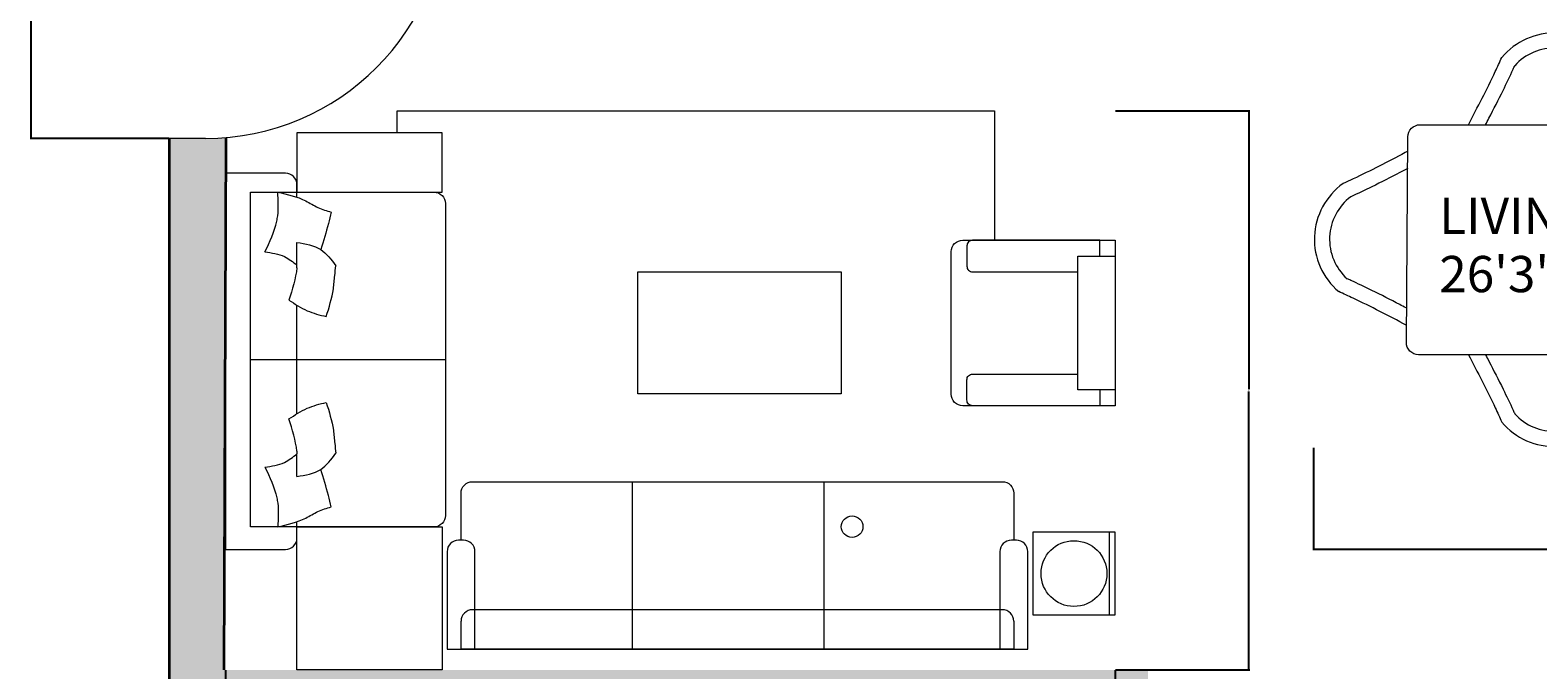
# Model space of a CAD drawing. Units: inches. Extents: x 1789 to 2841, y 3180 to 3702.
# Tile 10 of 14: x 2374 to 2624, y 3385 to 3491. Entities that reach past the tile are written whole.
import ezdxf

# ---------------------------------------------------------------- set-up
doc = ezdxf.new("R2010")
doc.units = ezdxf.units.IN
doc.header["$MEASUREMENT"] = 0
for name, color, linetype, lineweight in [('A-ANNO-DIMS', 2, 'Continuous', 18), ('A-AREA-IDEN', 7, 'Continuous', 18), ('A-WALL', 40, 'Continuous', 35), ('A-WALL-PATT', 252, 'Continuous', 13), ('DORS', 70, 'Continuous', 18), ('FURNITURE', 34, 'Continuous', 18)]:
    doc.layers.add(name, color=color, linetype=linetype, lineweight=lineweight)
doc.styles.get("Standard").update_dxf_attribs({"font": 'arial.ttf'})
doc.dimstyles.get("Standard").update_dxf_attribs({"dimtxt": 0.18, "dimasz": 0.18, "dimexe": 0.18, "dimexo": 0.0625, "dimgap": 0.09, "dimtad": 0, "dimtih": 1, "dimtoh": 1, "dimdec": 0, "dimzin": 0, "dimdsep": 46, "dimlunit": 3, "dimtxsty": 'Standard', "dimcen": 0.09, "dimadec": 0, "dimazin": 0, "dimtfac": 1, "dimtdec": 0, "dimtofl": 0, "dimtmove": 0, "dimatfit": 3, "dimfxl": 1, "dimtolj": 1, "dimtzin": 0, "dimarcsym": 0})

# ---------------------------------------------------------------- blocks, each defined once
blk = doc.blocks.new('SOFA')
for p, q in [((2185.57, 3479.13), (2185.57, 3482.99)), ((2185.57, 3482.99), (2290.09, 3482.99)), ((2290.09, 3482.99), (2290.09, 3460.33)), ((2159.93, 3439.46), (2194.03, 3439.46)), ((2226.79, 3388.76), (2226.79, 3418.07)), ((2260.29, 3388.76), (2260.29, 3418.07)), ((2310.14, 3409.22), (2310.14, 3394.77))]:
    blk.add_line(p, q)
for points in [[(2168.05, 3468.75), (2193.44, 3468.75), (2193.44, 3479.13), (2168.05, 3479.13)], [(2304.69, 3457.56), (2311.21, 3457.56), (2311.21, 3434.14), (2304.69, 3434.14)], [(2227.7, 3454.8), (2263.24, 3454.8), (2263.24, 3433.45), (2227.7, 3433.45)], [(2168.05, 3410.16), (2193.44, 3410.16), (2193.44, 3385.14), (2168.05, 3385.14)], [(2296.77, 3394.77), (2311.21, 3394.77), (2311.21, 3409.22), (2296.77, 3409.22)]]:
    blk.add_lwpolyline(points, close=True)
for points in [[(2168.05, 3467.86), (2168.05, 3470.06, 0.414214), (2166.05, 3472.06), (2155.57, 3472.06), (2155.57, 3406.2), (2166.05, 3406.2, 0.414214), (2168.05, 3408.2), (2168.05, 3411.06)], [(2308.49, 3457.56), (2308.49, 3460.33), (2286.26, 3460.33, 0.414214), (2285.26, 3459.33), (2285.26, 3455.79, 0.414214), (2286.26, 3454.79), (2304.69, 3454.79)], [(2308.49, 3434.14), (2308.49, 3431.37), (2286.26, 3431.37, -0.414214), (2285.26, 3432.37), (2285.26, 3435.9, -0.414214), (2286.26, 3436.9), (2304.69, 3436.9)], [(2196.77, 3407.83), (2196.77, 3416.07, -0.414214), (2198.77, 3418.07), (2291.47, 3418.07, -0.414214), (2293.47, 3416.07), (2293.47, 3407.83)], [(2293.47, 3393.66, 0.414214), (2291.47, 3395.66), (2198.77, 3395.66, 0.414214), (2196.77, 3393.66)]]:
    blk.add_lwpolyline(points, format="xyb")
for points in [[(2159.93, 3468.75), (2192.03, 3468.75, -0.414214), (2194.03, 3466.75), (2194.03, 3412.16, -0.414214), (2192.03, 3410.16), (2159.93, 3410.16)], [(2284.53, 3460.33), (2311.21, 3460.33), (2311.21, 3431.37), (2284.53, 3431.37, -0.414214), (2282.53, 3433.37), (2282.53, 3458.33, -0.414214)], [(2197.2, 3407.83), (2196.33, 3407.83, 0.414214), (2194.33, 3405.83), (2194.33, 3388.76), (2199.2, 3388.76), (2199.2, 3405.83, 0.414214)], [(2293.91, 3407.83), (2293.04, 3407.83, 0.414214), (2291.04, 3405.83), (2291.04, 3388.76), (2295.91, 3388.76), (2295.91, 3405.83, 0.414214)]]:
    blk.add_lwpolyline(points, format="xyb", close=True)
for points in [[(2168.05, 3455.52), (2168.05, 3459.94)], [(2168.05, 3429.95), (2168.05, 3448.97)], [(2168.05, 3423.4), (2168.05, 3422.93)], [(2168.05, 3418.98), (2168.05, 3422.93)], [(2293.47, 3393.66), (2293.47, 3388.76), (2196.77, 3388.76), (2196.77, 3393.66)], [(2196.77, 3388.76), (2293.47, 3388.76)]]:
    blk.add_lwpolyline(points)
for centre, radius in [((2265.18, 3410.2), 1.89), ((2303.99, 3401.99), 5.76)]:
    blk.add_circle(centre, radius)
for points, knots in [([(2162.46, 3458.3), (2163.29, 3460.04), (2164.26, 3462.07), (2164.89, 3465.65), (2164.78, 3467.36), (2164.69, 3468.75)], [0, 0, 0, 0, 5.733795, 6.696566, 10.854822, 10.854822, 10.854822, 10.854822]), ([(2164.69, 3468.75), (2166.38, 3468.37), (2168.87, 3467.8), (2171.7, 3465.95), (2173.26, 3465.49), (2174.05, 3465.25)], [0, 0, 0, 0, 5.14676, 7.56322, 10.027291, 10.027291, 10.027291, 10.027291]), ([(2174.05, 3465.25), (2173.89, 3464.58), (2173.37, 3462.38), (2172.69, 3460.22), (2172.22, 3458.71)], [0, 0, 0, 0, 2.055182, 6.796603, 6.796603, 6.796603, 6.796603]), ([(2162.46, 3458.3), (2163.64, 3458.13), (2165.71, 3457.83), (2167.35, 3456.54), (2168.05, 3455.99)], [0, 0, 0, 0, 3.512009, 6.140853, 6.140853, 6.140853, 6.140853]), ([(2168.05, 3459.94), (2169.55, 3459.7), (2172.38, 3459.25), (2174.06, 3456.94), (2174.85, 3455.84)], [0, 0, 0, 0, 4.35123, 8.24052, 8.24052, 8.24052, 8.24052]), ([(2173.18, 3446.97), (2173.68, 3448.57), (2174.42, 3450.93), (2174.65, 3453.95), (2174.79, 3455.29), (2174.85, 3455.84)], [0, 0, 0, 0, 5.016146, 7.373936, 9.056838, 9.056838, 9.056838, 9.056838]), ([(2166.66, 3449.86), (2167.7, 3449.17), (2169.71, 3447.85), (2172.05, 3447.25), (2173.18, 3446.97)], [0, 0, 0, 0, 3.710874, 7.178588, 7.178588, 7.178588, 7.178588]), ([(2166.66, 3429.05), (2167.7, 3429.74), (2169.71, 3431.07), (2172.05, 3431.66), (2173.18, 3431.95)], [0, 0, 0, 0, 3.710874, 7.178588, 7.178588, 7.178588, 7.178588]), ([(2173.18, 3431.95), (2173.68, 3430.35), (2174.42, 3427.99), (2174.65, 3424.97), (2174.79, 3423.63), (2174.85, 3423.07)], [0, 0, 0, 0, 5.016146, 7.373936, 9.056838, 9.056838, 9.056838, 9.056838]), ([(2162.46, 3420.62), (2163.64, 3420.79), (2165.71, 3421.09), (2167.35, 3422.37), (2168.05, 3422.93)], [0, 0, 0, 0, 3.512009, 6.140853, 6.140853, 6.140853, 6.140853]), ([(2168.05, 3418.98), (2169.55, 3419.22), (2172.38, 3419.66), (2174.06, 3421.98), (2174.85, 3423.07)], [0, 0, 0, 0, 4.35123, 8.24052, 8.24052, 8.24052, 8.24052]), ([(2162.46, 3420.62), (2163.29, 3418.88), (2164.26, 3416.85), (2164.89, 3413.27), (2164.78, 3411.56), (2164.69, 3410.16)], [0, 0, 0, 0, 5.733795, 6.696566, 10.854822, 10.854822, 10.854822, 10.854822]), ([(2174.05, 3413.67), (2173.89, 3414.33), (2173.37, 3416.54), (2172.69, 3418.7), (2172.22, 3420.21)], [0, 0, 0, 0, 2.055182, 6.796603, 6.796603, 6.796603, 6.796603]), ([(2164.69, 3410.16), (2166.38, 3410.55), (2168.87, 3411.12), (2171.7, 3412.96), (2173.26, 3413.43), (2174.05, 3413.67)], [0, 0, 0, 0, 5.14676, 7.56322, 10.027291, 10.027291, 10.027291, 10.027291])]:
    blk.add_open_spline(points, degree=3, knots=knots)
for points in [[(2168.05, 3455.52), (2167.85, 3453.6), (2167.25, 3451.73), (2166.66, 3449.86)], [(2168.05, 3423.4), (2167.85, 3425.31), (2167.25, 3427.18), (2166.66, 3429.05)]]:
    blk.add_open_spline(points, degree=3)
blk = doc.blocks.new('DINI')
blk.add_lwpolyline([(2038.22, 3475.42), (2115.97, 3475.42, -0.414214), (2117.97, 3473.42), (2117.72, 3439.35, -0.414214), (2115.72, 3437.35), (2037.97, 3437.35, -0.414214), (2035.97, 3439.35), (2036.22, 3473.42, -0.414214)], format="xyb", close=True)
for centre, radius, start, end in [((2060.43, 3479.31), 11.31, 35.4017, 140.0736), ((2093.76, 3479.31), 11.31, 39.9264, 144.5983), ((2060.43, 3479.31), 8.8, 36.8657, 137.9611), ((2093.76, 3479.31), 8.8, 42.0389, 143.1343), ((2032.05, 3456.46), 11.31, 125.4017, 230.0736), ((2032.05, 3456.46), 8.8, 126.8657, 227.9611), ((2121.64, 3456.46), 8.8, 312.0389, 53.1343), ((2121.64, 3456.46), 11.31, 309.9264, 54.5983), ((2060.43, 3433.45), 11.31, 219.9264, 324.5983), ((2060.43, 3433.45), 8.8, 222.0389, 323.1343), ((2093.76, 3433.45), 11.31, 215.4017, 320.0736), ((2093.76, 3433.45), 8.8, 216.8657, 317.9611)]:
    blk.add_arc(centre, radius, start, end)
for points, knots in [([(2046.22, 3475.42), (2047.75, 3478.33), (2049.68, 3482.01), (2051.4, 3485.79), (2051.76, 3486.58)], [0, 0, 0, 0, 7.856931, 9.915256, 9.915256, 9.915256, 9.915256]), ([(2107.98, 3475.42), (2106.45, 3478.33), (2104.51, 3482.01), (2102.79, 3485.79), (2102.44, 3486.58)], [0, 0, 0, 0, 7.856931, 9.915256, 9.915256, 9.915256, 9.915256]), ([(2049.05, 3475.42), (2049.25, 3475.79), (2049.44, 3476.15), (2050.42, 3478.03), (2051.21, 3479.56), (2052.54, 3482.27), (2053.1, 3483.45), (2053.72, 3484.82), (2053.81, 3485.01), (2053.9, 3485.21)], [1.048693, 1.048693, 1.048693, 1.048693, 2.029233, 2.029233, 6.0877, 6.0877, 9.118148, 9.118148, 9.624349, 9.624349, 9.624349, 9.624349]), ([(2072.04, 3475.42), (2071.85, 3475.78), (2071.66, 3476.15), (2070.68, 3478.03), (2069.89, 3479.55), (2068.56, 3482.26), (2068.01, 3483.43), (2067.48, 3484.59)], [1.048889, 1.048889, 1.048889, 1.048889, 2.02655, 2.02655, 6.079649, 6.079649, 9.095857, 9.095857, 9.095857, 9.095857]), ([(2074.88, 3475.42), (2073.35, 3478.33), (2071.54, 3481.78), (2069.91, 3485.32), (2069.66, 3485.87)], [0, 0, 0, 0, 7.856931, 9.297576, 9.297576, 9.297576, 9.297576]), ([(2079.31, 3475.42), (2080.85, 3478.33), (2082.66, 3481.78), (2084.29, 3485.32), (2084.54, 3485.87)], [0, 0, 0, 0, 7.856931, 9.297576, 9.297576, 9.297576, 9.297576]), ([(2082.15, 3475.42), (2082.34, 3475.78), (2082.53, 3476.15), (2083.51, 3478.03), (2084.3, 3479.55), (2085.63, 3482.26), (2086.19, 3483.43), (2086.72, 3484.59)], [1.048889, 1.048889, 1.048889, 1.048889, 2.02655, 2.02655, 6.079649, 6.079649, 9.095857, 9.095857, 9.095857, 9.095857]), ([(2105.14, 3475.42), (2104.95, 3475.79), (2104.76, 3476.15), (2103.78, 3478.03), (2102.99, 3479.56), (2101.65, 3482.27), (2101.1, 3483.45), (2100.47, 3484.82), (2100.38, 3485.01), (2100.3, 3485.21)], [1.048693, 1.048693, 1.048693, 1.048693, 2.029233, 2.029233, 6.0877, 6.0877, 9.118148, 9.118148, 9.624349, 9.624349, 9.624349, 9.624349]), ([(2036.2, 3471.04), (2036.05, 3470.96), (2035.89, 3470.88), (2035.74, 3470.8), (2035.74, 3470.8), (2035.74, 3470.8), (2035.74, 3470.8), (2032.89, 3469.3), (2029.51, 3467.53), (2026.05, 3465.93), (2025.5, 3465.68)], [-0.229823, -0.229823, -0.229823, -0.229823, 0.189373, 0.189373, 0.189373, 0.189712, 0.189712, 0.189712, 7.856931, 9.297576, 9.297576, 9.297576, 9.297576]), ([(2117.95, 3470.8), (2120.8, 3469.3), (2124.18, 3467.53), (2127.64, 3465.93), (2128.19, 3465.68)], [0.189712, 0.189712, 0.189712, 0.189712, 7.856931, 9.297576, 9.297576, 9.297576, 9.297576]), ([(2036.18, 3468.19), (2036.04, 3468.12), (2035.9, 3468.04), (2035.76, 3467.97), (2035.76, 3467.97), (2035.76, 3467.97), (2035.76, 3467.97), (2035.46, 3467.81), (2035.16, 3467.65), (2033.34, 3466.71), (2031.81, 3465.92), (2029.11, 3464.59), (2027.94, 3464.04), (2026.77, 3463.5)], [0.838882, 0.838882, 0.838882, 0.838882, 1.215073, 1.215073, 1.215073, 1.219193, 1.219193, 1.219193, 2.02655, 2.02655, 6.079649, 6.079649, 9.095857, 9.095857, 9.095857, 9.095857]), ([(2117.93, 3467.97), (2118.23, 3467.81), (2118.53, 3467.65), (2120.35, 3466.71), (2121.88, 3465.92), (2124.58, 3464.59), (2125.75, 3464.04), (2126.92, 3463.5)], [1.219193, 1.219193, 1.219193, 1.219193, 2.02655, 2.02655, 6.079649, 6.079649, 9.095857, 9.095857, 9.095857, 9.095857]), ([(2035.95, 3445.08), (2035.58, 3445.27), (2035.22, 3445.46), (2033.34, 3446.45), (2031.81, 3447.23), (2029.1, 3448.57), (2027.92, 3449.12), (2026.55, 3449.75), (2026.36, 3449.84), (2026.16, 3449.93)], [1.048693, 1.048693, 1.048693, 1.048693, 2.029233, 2.029233, 6.0877, 6.0877, 9.118148, 9.118148, 9.624349, 9.624349, 9.624349, 9.624349]), ([(2117.74, 3445.08), (2118.11, 3445.27), (2118.47, 3445.46), (2120.35, 3446.45), (2121.88, 3447.23), (2124.59, 3448.57), (2125.77, 3449.12), (2127.14, 3449.75), (2127.33, 3449.84), (2127.53, 3449.93)], [1.048693, 1.048693, 1.048693, 1.048693, 2.029233, 2.029233, 6.0877, 6.0877, 9.118148, 9.118148, 9.624349, 9.624349, 9.624349, 9.624349]), ([(2035.95, 3442.24), (2033.03, 3443.77), (2029.36, 3445.71), (2025.58, 3447.43), (2024.79, 3447.79)], [0, 0, 0, 0, 7.856931, 9.915256, 9.915256, 9.915256, 9.915256]), ([(2117.74, 3442.24), (2120.66, 3443.77), (2124.33, 3445.71), (2128.11, 3447.43), (2128.9, 3447.79)], [0, 0, 0, 0, 7.856931, 9.915256, 9.915256, 9.915256, 9.915256]), ([(2046.22, 3437.35), (2047.75, 3434.43), (2049.68, 3430.75), (2051.4, 3426.98), (2051.76, 3426.19)], [0, 0, 0, 0, 7.856931, 9.915256, 9.915256, 9.915256, 9.915256]), ([(2049.05, 3437.35), (2049.25, 3436.98), (2049.44, 3436.62), (2050.42, 3434.73), (2051.21, 3433.2), (2052.54, 3430.5), (2053.1, 3429.32), (2053.72, 3427.95), (2053.81, 3427.75), (2053.9, 3427.56)], [1.048693, 1.048693, 1.048693, 1.048693, 2.029233, 2.029233, 6.0877, 6.0877, 9.118148, 9.118148, 9.624349, 9.624349, 9.624349, 9.624349]), ([(2072.04, 3437.35), (2071.85, 3436.98), (2071.66, 3436.62), (2070.68, 3434.74), (2069.89, 3433.21), (2068.56, 3430.51), (2068.01, 3429.34), (2067.48, 3428.17)], [1.048889, 1.048889, 1.048889, 1.048889, 2.02655, 2.02655, 6.079649, 6.079649, 9.095857, 9.095857, 9.095857, 9.095857]), ([(2074.88, 3437.35), (2073.35, 3434.43), (2071.54, 3430.98), (2069.91, 3427.45), (2069.66, 3426.9)], [0, 0, 0, 0, 7.856931, 9.297576, 9.297576, 9.297576, 9.297576]), ([(2079.31, 3437.35), (2080.85, 3434.43), (2082.66, 3430.98), (2084.29, 3427.45), (2084.54, 3426.9)], [0, 0, 0, 0, 7.856931, 9.297576, 9.297576, 9.297576, 9.297576]), ([(2082.15, 3437.35), (2082.34, 3436.98), (2082.53, 3436.62), (2083.51, 3434.74), (2084.3, 3433.21), (2085.63, 3430.51), (2086.19, 3429.34), (2086.72, 3428.17)], [1.048889, 1.048889, 1.048889, 1.048889, 2.02655, 2.02655, 6.079649, 6.079649, 9.095857, 9.095857, 9.095857, 9.095857]), ([(2105.14, 3437.35), (2104.95, 3436.98), (2104.76, 3436.62), (2103.78, 3434.73), (2102.99, 3433.2), (2101.65, 3430.5), (2101.1, 3429.32), (2100.47, 3427.95), (2100.38, 3427.75), (2100.3, 3427.56)], [1.048693, 1.048693, 1.048693, 1.048693, 2.029233, 2.029233, 6.0877, 6.0877, 9.118148, 9.118148, 9.624349, 9.624349, 9.624349, 9.624349]), ([(2107.98, 3437.35), (2106.45, 3434.43), (2104.51, 3430.75), (2102.79, 3426.98), (2102.44, 3426.19)], [0, 0, 0, 0, 7.856931, 9.915256, 9.915256, 9.915256, 9.915256])]:
    blk.add_open_spline(points, degree=3, knots=knots)
blk = doc.blocks.new('*U26')
for p, q in [((0, 0), (0, -6)), ((40, 0), (40, -6))]:
    blk.add_line(p, q)
blk.add_lwpolyline([(0, 0), (0, 40), (1.75, 40), (1.75, 0)], close=True)
blk.add_arc((0, 0), 40, 0, 90)
blk = doc.blocks.new('*D69')
at = {"layer": 'A-ANNO-DIMS', "color": 0, "lineweight": -2, "transparency": 16777216}
for p, q in [((2406.54, 3385.11), (2406.54, 3362.9)), ((2553.79, 3385.11), (2553.79, 3362.9)), ((2406.72, 3363.08), (2478.8, 3363.08)), ((2553.61, 3363.08), (2481.54, 3363.08))]:
    blk.add_line(p, q, dxfattribs=at)
at = {"layer": 'A-ANNO-DIMS', "color": 0, "transparency": 16777216}
for points in [[(2406.72, 3363.11), (2406.72, 3363.05), (2406.54, 3363.08)], [(2553.61, 3363.11), (2553.61, 3363.05), (2553.79, 3363.08)]]:
    blk.add_solid(points, dxfattribs=at)
at = {"layer": 'Defpoints', "color": 0, "transparency": 16777216}
for p in [(2406.54, 3385.17), (2553.79, 3385.17), (2553.79, 3363.08)]:
    blk.add_point(p, dxfattribs=at)
at = {"layer": 'A-ANNO-DIMS', "color": 0, "transparency": 16777216, "insert": (2480.17, 3363.08), "char_height": 0.18, "attachment_point": 5}
blk.add_mtext('\\A1;SEATING GROUP 147', dxfattribs=at)
blk = doc.blocks.new('*D70')
at = {"layer": 'A-ANNO-DIMS', "color": 0, "lineweight": -2, "transparency": 16777216}
for p, q in [((2553.85, 3477.74), (2576.06, 3477.74)), ((2575.88, 3477.56), (2575.88, 3431.63)), ((2575.88, 3385.35), (2575.88, 3431.27)), ((2553.85, 3385.17), (2576.06, 3385.17))]:
    blk.add_line(p, q, dxfattribs=at)
at = {"layer": 'A-ANNO-DIMS', "color": 0, "transparency": 16777216}
for points in [[(2575.85, 3477.56), (2575.91, 3477.56), (2575.88, 3477.74)], [(2575.85, 3385.35), (2575.91, 3385.35), (2575.88, 3385.17)]]:
    blk.add_solid(points, dxfattribs=at)
at = {"layer": 'Defpoints', "color": 0, "transparency": 16777216}
for p in [(2553.79, 3477.74), (2575.88, 3477.74), (2553.79, 3385.17)]:
    blk.add_point(p, dxfattribs=at)
at = {"layer": 'A-ANNO-DIMS', "color": 0, "transparency": 16777216, "insert": (2575.88, 3431.45), "char_height": 0.18, "attachment_point": 5}
blk.add_mtext('\\A1;93', dxfattribs=at)
blk = doc.blocks.new('*D71')
at = {"layer": 'A-ANNO-DIMS', "color": 0, "lineweight": -2, "transparency": 16777216}
for p, q in [((2586.62, 3421.95), (2586.62, 3404.96)), ((2699.09, 3421.95), (2699.09, 3404.96)), ((2586.8, 3405.14), (2641.51, 3405.14)), ((2698.91, 3405.14), (2644.2, 3405.14))]:
    blk.add_line(p, q, dxfattribs=at)
at = {"layer": 'A-ANNO-DIMS', "color": 0, "transparency": 16777216}
for points in [[(2586.8, 3405.17), (2586.8, 3405.11), (2586.62, 3405.14)], [(2698.91, 3405.17), (2698.91, 3405.11), (2699.09, 3405.14)]]:
    blk.add_solid(points, dxfattribs=at)
at = {"layer": 'Defpoints', "color": 0, "transparency": 16777216}
for p in [(2586.62, 3422.01), (2699.09, 3422.01), (2699.09, 3405.14)]:
    blk.add_point(p, dxfattribs=at)
at = {"layer": 'A-ANNO-DIMS', "color": 0, "transparency": 16777216, "insert": (2642.85, 3405.14), "char_height": 0.18, "attachment_point": 5}
blk.add_mtext('\\A1;DINING SET 112 TYP.', dxfattribs=at)
blk = doc.blocks.new('*D104')
at = {"layer": 'A-ANNO-DIMS', "color": 0, "lineweight": -2, "transparency": 16777216}
for p, q in [((2397.17, 3513.16), (2374.2, 3513.16)), ((2374.38, 3512.98), (2374.38, 3493.34)), ((2374.38, 3473.34), (2374.38, 3492.98)), ((2397.17, 3473.16), (2374.2, 3473.16))]:
    blk.add_line(p, q, dxfattribs=at)
at = {"layer": 'A-ANNO-DIMS', "color": 0, "transparency": 16777216}
for points in [[(2374.35, 3512.98), (2374.41, 3512.98), (2374.38, 3513.16)], [(2374.35, 3473.34), (2374.41, 3473.34), (2374.38, 3473.16)]]:
    blk.add_solid(points, dxfattribs=at)
at = {"layer": 'Defpoints', "color": 0, "transparency": 16777216}
for p in [(2397.23, 3513.16), (2374.38, 3473.16), (2397.23, 3473.16)]:
    blk.add_point(p, dxfattribs=at)
at = {"layer": 'A-ANNO-DIMS', "color": 0, "transparency": 16777216, "insert": (2374.38, 3493.16), "char_height": 0.18, "attachment_point": 5}
blk.add_mtext('\\A1;40', dxfattribs=at)

msp = doc.modelspace()

# ---------------------------------------------------------------- hatches: boundary and pattern name
at = {"layer": 'A-WALL-PATT'}
h = msp.add_hatch(color=256, dxfattribs=at)
h.dxf.hatch_style = 1
edge = h.paths.add_edge_path()
edge.add_line((2559.2333, 3385.1608), (2442.3717, 3385.1608))
edge.add_line((2442.3717, 3385.1608), (2442.3717, 3385.1524))
edge.add_line((2442.3717, 3385.1524), (2418.8108, 3385.1608))
edge.add_line((2418.8108, 3385.1608), (2406.2333, 3385.1608))
edge.add_line((2406.2333, 3385.1608), (2406.5667, 3473.2999))
edge.add_arc((2403.2333, 3513.1608), 40, 270, 274.780192, ccw=False)
edge.add_line((2403.2333, 3473.1608), (2397.2333, 3473.1608))
edge.add_line((2397.2333, 3473.1608), (2397.2333, 3376.1608))
edge.add_line((2397.2333, 3376.1608), (2550.2333, 3376.1608))
edge.add_line((2550.2333, 3376.1608), (2550.2333, 3372.6905))
edge.add_arc((2551.7333, 3408.5966), 35.9374, 267.607822, 272.392178)
edge.add_line((2553.2333, 3372.6905), (2559.2333, 3372.6905))
edge.add_line((2559.2333, 3372.6905), (2559.2333, 3385.1608))

# ---------------------------------------------------------------- linework, layer by layer
at = {"layer": 'A-WALL'}
for p, q in [((2397.2333, 3473.1608), (2397.2333, 3203.1608)), ((2406.5667, 3473.2999), (2406.2333, 3385.1608))]:
    msp.add_line(p, q, dxfattribs=at)

# ---------------------------------------------------------------- block references
at = {"layer": 'DORS', "rotation": 270}
msp.add_blockref('*U26', (2403.2333, 3513.1608), dxfattribs=at)
at = {"layer": 'FURNITURE'}
msp.add_blockref('DINI', (566.0099, 0), dxfattribs=at)
at = {"layer": 'FURNITURE', "xscale": 0.946071628049247, "yscale": 0.946071628049247, "zscale": 0.946071628049247}
msp.add_blockref('SOFA', (367.219, 182.5797), dxfattribs=at)

# ---------------------------------------------------------------- texts
at = {"layer": 'A-ANNO-DIMS'}
msp.add_text("26'3''X11'0''", height=6, dxfattribs=at).set_placement((2607.4196, 3447.6999))
at = {"layer": 'A-AREA-IDEN'}
msp.add_text('LIVING&DRAWING', height=6, dxfattribs=at).set_placement((2607.4196, 3457.3383))

# ---------------------------------------------------------------- dimensions: what is measured, and where the dimension line sits
at = {"layer": 'A-ANNO-DIMS'}
for base, p1, p2, picture, middle in [((2374.3833, 3473.1608), (2397.2333, 3513.1608), (2397.2333, 3473.1608), '*D104', (2374.3833, 3493.1608)), ((2575.8765, 3477.7369), (2553.7897, 3385.1685), (2553.7897, 3477.7369), '*D70', (2575.8765, 3431.4527))]:
    dim = msp.add_linear_dim(base=base, p1=p1, p2=p2, angle=90, dimstyle='Standard', override={"dimdec": 0, "dimlfac": 1, "dimrnd": 0, "dimzin": 0, "dimdsep": 46, "dimlunit": 2}, dxfattribs=at)
    dim.commit()
    dim.dimension.update_dxf_attribs({"geometry": picture, "text_midpoint": middle})
for base, p1, p2, text, picture, middle in [((2699.0888, 3405.1391), (2586.621, 3422.0092), (2699.0888, 3422.0092), 'DINING SET <> TYP.', '*D71', (2642.8549, 3405.1391)), ((2553.7897, 3363.0817), (2406.5443, 3385.1685), (2553.7897, 3385.1685), 'SEATING GROUP <>', '*D69', (2480.167, 3363.0817))]:
    dim = msp.add_linear_dim(base=base, p1=p1, p2=p2, text=text, dimstyle='Standard', override={"dimdec": 0, "dimlfac": 1, "dimrnd": 0, "dimzin": 0, "dimdsep": 46, "dimlunit": 2}, dxfattribs=at)
    dim.commit()
    dim.dimension.update_dxf_attribs({"geometry": picture, "text_midpoint": middle})

doc.saveas('drawing.dxf')
